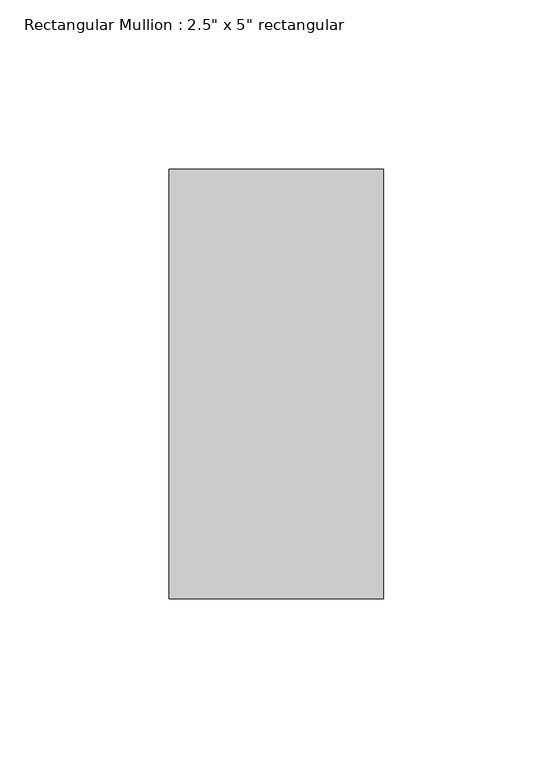
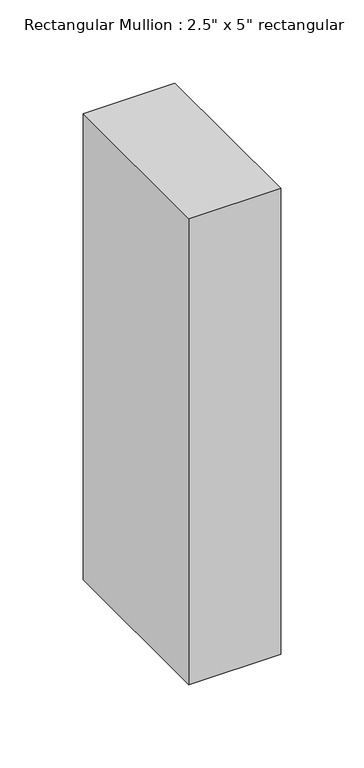
"""IFC4 building model written with IfcOpenShell, lengths in millimetres: member geometry."""

from ifc_helpers import new_model, si_unit, frame, origin, place, context, project, spatial, polyline, outline, extrude, source, transform, mapped, element, save


def member_5ca2be8d(model_context):
    return source(origin(), model_context, "Body", "SweptSolid", [
        extrude(outline(polyline([(0.0, 63.5), (0.0, -63.5), (-63.5, -63.5), (-63.5, 63.5), (0.0, 63.5)])), frame((0.0, 0.0, -341.8283762), z_axis=(0.0, 0.0, 1.0), x_axis=(1.0, 0.0, 0.0)), (0.0, 0.0, 1.0), 341.8283762),
    ])


if __name__ == "__main__":
    model = new_model("IFC4")
    model_context = context("Model", 3, world=origin())
    ifc_project = project(units=[si_unit("LENGTHUNIT", "METRE", prefix="MILLI")], contexts=[model_context])
    site = spatial("IfcSite", under=ifc_project)
    building = spatial("IfcBuilding", under=site)
    placement = place(None, origin())
    member_shape = member_5ca2be8d(model_context)
    element("IfcMember", 1, ObjectType="Rectangular Mullion : 2.5\" x 5\" rectangular", at=placement, inside=building, context=model_context, shape_type="MappedRepresentation", body=[
        mapped(member_shape, transform((0.0, 0.0, 0.0), x_axis=(1.0, 0.0, 0.0), y_axis=(0.0, 1.0, 0.0), z_axis=(0.0, 0.0, 1.0))),
    ])
    save(model, "model.ifc")

# Revit data of these elements
# Type "Rectangular Mullion : 2.5\" x 5\" rectangular"
#   built-in parameter 1007304 = 0.416667 (stored number, unit not read)
#   built-in parameter 1007301 = 0.104167 (stored number, unit not read)
#   built-in parameter 1007300 = 0.104167 (stored number, unit not read)
# Element 1 (IfcMember, "Rectangular Mullion : 2.5\" x 5\" rectangular")
#   Materials on its faces: "Aluminum"
# Materials
#   "Aluminum": class "Metal", colour RGB 247 247 247, transparency 0, Description = "Aluminum 6061", Cost = 0
